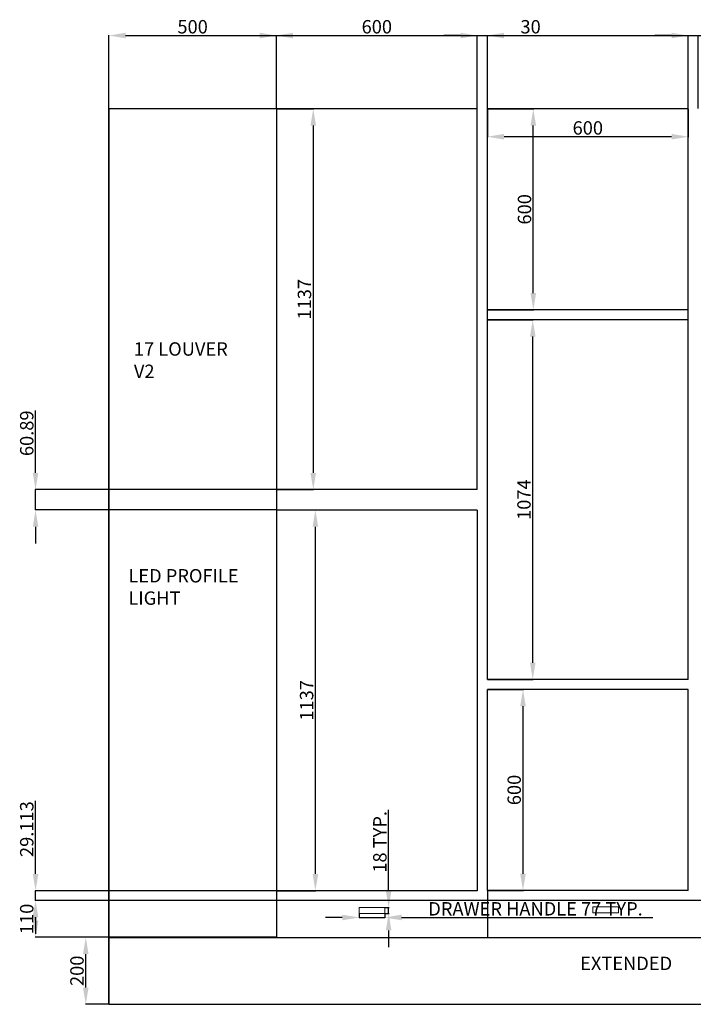
# Model space of a CAD drawing. Units: millimetres. Extents: x -2182 to 7969, y 257 to 4097.
# Tile 1 of 5: x -2182 to -171, y 508 to 3449. Entities that reach past the tile are written whole.
import ezdxf

# ---------------------------------------------------------------- set-up
doc = ezdxf.new("R2010")
doc.units = ezdxf.units.MM
for name, color, linetype, lineweight in [('A-ANNO-DIMS', 2, 'Continuous', 18), ('A-ANNO-TEXT', 3, 'Continuous', 18), ('A-ELEV', 7, 'Continuous', 25), ('A-FURN-HRDW', 8, 'Continuous', 18)]:
    doc.layers.add(name, color=color, linetype=linetype, lineweight=lineweight)
doc.styles.get("Standard").update_dxf_attribs({"font": 'arial.ttf'})
doc.dimstyles.new('ISO-25', dxfattribs={"dimtxt": 40, "dimasz": 50, "dimexe": 1.25, "dimexo": 0.625, "dimtad": 1, "dimtxsty": 'Standard', "dimcen": 2.5, "dimadec": 0, "dimazin": 0, "dimtfac": 1, "dimtmove": 0, "dimatfit": 3, "dimfxl": 1, "dimarcsym": 0})

# ---------------------------------------------------------------- blocks, each defined once
blk = doc.blocks.new('*D24')
at = {"layer": 'A-ANNO-DIMS', "color": 0, "lineweight": -2, "transparency": 16777216}
for p, q in [((-785.2, 1448.5), (-678.1, 1448.5)), ((-679.3, 898.5), (-679.3, 1398.5)), ((-785.2, 848.5), (-678.1, 848.5))]:
    blk.add_line(p, q, dxfattribs=at)
at = {"layer": 'A-ANNO-DIMS', "color": 0, "transparency": 16777216}
for points in [[(-687.7, 1398.5), (-671, 1398.5), (-679.3, 1448.5)], [(-687.7, 898.5), (-671, 898.5), (-679.3, 848.5)]]:
    blk.add_solid(points, dxfattribs=at)
at = {"layer": 'Defpoints', "color": 0, "transparency": 16777216}
for p in [(-785.8, 1448.5), (-679.3, 1448.5), (-785.8, 848.5)]:
    blk.add_point(p, dxfattribs=at)
at = {"layer": 'A-ANNO-DIMS', "color": 0, "transparency": 16777216, "insert": (-700.4, 1148.5), "char_height": 40, "attachment_point": 5, "rotation": 90}
blk.add_mtext('600', dxfattribs=at)
blk = doc.blocks.new('*D25')
at = {"layer": 'A-ANNO-DIMS', "color": 0, "lineweight": -2, "transparency": 16777216}
for p, q in [((-785.2, 2552.5), (-648.9, 2552.5)), ((-650.2, 1528.5), (-650.2, 2502.5)), ((-785.2, 1478.5), (-648.9, 1478.5))]:
    blk.add_line(p, q, dxfattribs=at)
at = {"layer": 'A-ANNO-DIMS', "color": 0, "transparency": 16777216}
for points in [[(-658.5, 2502.5), (-641.9, 2502.5), (-650.2, 2552.5)], [(-658.5, 1528.5), (-641.9, 1528.5), (-650.2, 1478.5)]]:
    blk.add_solid(points, dxfattribs=at)
at = {"layer": 'Defpoints', "color": 0, "transparency": 16777216}
for p in [(-785.8, 2552.5), (-650.2, 2552.5), (-785.8, 1478.5)]:
    blk.add_point(p, dxfattribs=at)
at = {"layer": 'A-ANNO-DIMS', "color": 0, "transparency": 16777216, "insert": (-671.2, 2015.5), "char_height": 40, "attachment_point": 5, "rotation": 90}
blk.add_mtext('1074', dxfattribs=at)
blk = doc.blocks.new('*D26')
at = {"layer": 'A-ANNO-DIMS', "color": 0, "lineweight": -2, "transparency": 16777216}
for p, q in [((-785.2, 3182.5), (-647.3, 3182.5)), ((-648.5, 2632.5), (-648.5, 3132.5)), ((-785.2, 2582.5), (-647.3, 2582.5))]:
    blk.add_line(p, q, dxfattribs=at)
at = {"layer": 'A-ANNO-DIMS', "color": 0, "transparency": 16777216}
for points in [[(-656.9, 3132.5), (-640.2, 3132.5), (-648.5, 3182.5)], [(-656.9, 2632.5), (-640.2, 2632.5), (-648.5, 2582.5)]]:
    blk.add_solid(points, dxfattribs=at)
at = {"layer": 'Defpoints', "color": 0, "transparency": 16777216}
for p in [(-785.8, 3182.5), (-648.5, 3182.5), (-785.8, 2582.5)]:
    blk.add_point(p, dxfattribs=at)
at = {"layer": 'A-ANNO-DIMS', "color": 0, "transparency": 16777216, "insert": (-669.6, 2882.5), "char_height": 40, "attachment_point": 5, "rotation": 90}
blk.add_mtext('600', dxfattribs=at)
blk = doc.blocks.new('*D27')
at = {"layer": 'A-ANNO-DIMS', "color": 0, "lineweight": -2, "transparency": 16777216}
for p, q in [((-785.8, 3181.8), (-785.8, 3098.1)), ((-185.8, 3181.8), (-185.8, 3098.1)), ((-235.8, 3099.3), (-735.8, 3099.3))]:
    blk.add_line(p, q, dxfattribs=at)
at = {"layer": 'A-ANNO-DIMS', "color": 0, "transparency": 16777216}
for points in [[(-735.8, 3107.7), (-735.8, 3091), (-785.8, 3099.3)], [(-235.8, 3107.7), (-235.8, 3091), (-185.8, 3099.3)]]:
    blk.add_solid(points, dxfattribs=at)
at = {"layer": 'Defpoints', "color": 0, "transparency": 16777216}
for p in [(-785.8, 3182.5), (-185.8, 3182.5), (-785.8, 3099.3)]:
    blk.add_point(p, dxfattribs=at)
at = {"layer": 'A-ANNO-DIMS', "color": 0, "transparency": 16777216, "insert": (-485.8, 3120.4), "char_height": 40, "attachment_point": 5}
blk.add_mtext('600', dxfattribs=at)
blk = doc.blocks.new('*D28')
at = {"layer": 'A-ANNO-DIMS', "color": 0, "lineweight": -2, "transparency": 16777216}
for p, q in [((-1415.2, 3182.5), (-1304.4, 3182.5)), ((-1305.6, 3132.5), (-1305.6, 2095.5)), ((-1415.2, 2045.5), (-1304.4, 2045.5))]:
    blk.add_line(p, q, dxfattribs=at)
at = {"layer": 'A-ANNO-DIMS', "color": 0, "transparency": 16777216}
for points in [[(-1314, 3132.5), (-1297.3, 3132.5), (-1305.6, 3182.5)], [(-1314, 2095.5), (-1297.3, 2095.5), (-1305.6, 2045.5)]]:
    blk.add_solid(points, dxfattribs=at)
at = {"layer": 'Defpoints', "color": 0, "transparency": 16777216}
for p in [(-1415.8, 3182.5), (-1415.8, 2045.5), (-1305.6, 2045.5)]:
    blk.add_point(p, dxfattribs=at)
at = {"layer": 'A-ANNO-DIMS', "color": 0, "transparency": 16777216, "insert": (-1326.7, 2614), "char_height": 40, "attachment_point": 5, "rotation": 90}
blk.add_mtext('1137', dxfattribs=at)
blk = doc.blocks.new('*D29')
at = {"layer": 'A-ANNO-DIMS', "color": 0, "lineweight": -2, "transparency": 16777216}
for p, q in [((-1415.2, 1984.6), (-1297.9, 1984.6)), ((-1299.2, 897.6), (-1299.2, 1934.6)), ((-1415.2, 847.6), (-1297.9, 847.6))]:
    blk.add_line(p, q, dxfattribs=at)
at = {"layer": 'A-ANNO-DIMS', "color": 0, "transparency": 16777216}
for points in [[(-1307.5, 1934.6), (-1290.8, 1934.6), (-1299.2, 1984.6)], [(-1307.5, 897.6), (-1290.8, 897.6), (-1299.2, 847.6)]]:
    blk.add_solid(points, dxfattribs=at)
at = {"layer": 'Defpoints', "color": 0, "transparency": 16777216}
for p in [(-1415.8, 1984.6), (-1299.2, 1984.6), (-1415.8, 847.6)]:
    blk.add_point(p, dxfattribs=at)
at = {"layer": 'A-ANNO-DIMS', "color": 0, "transparency": 16777216, "insert": (-1320.2, 1416.1), "char_height": 40, "attachment_point": 5, "rotation": 90}
blk.add_mtext('1137', dxfattribs=at)
blk = doc.blocks.new('*D30')
at = {"layer": 'A-ANNO-DIMS', "color": 0, "lineweight": -2, "transparency": 16777216}
for p, q in [((-1916.4, 708.5), (-1986.1, 708.5)), ((-1984.8, 558.5), (-1984.8, 658.5)), ((-1916.4, 508.5), (-1986.1, 508.5))]:
    blk.add_line(p, q, dxfattribs=at)
at = {"layer": 'A-ANNO-DIMS', "color": 0, "transparency": 16777216}
for points in [[(-1993.2, 658.5), (-1976.5, 658.5), (-1984.8, 708.5)], [(-1993.2, 558.5), (-1976.5, 558.5), (-1984.8, 508.5)]]:
    blk.add_solid(points, dxfattribs=at)
at = {"layer": 'Defpoints', "color": 0, "transparency": 16777216}
for p in [(-1984.8, 708.5), (-1915.8, 708.5), (-1915.8, 508.5)]:
    blk.add_point(p, dxfattribs=at)
at = {"layer": 'A-ANNO-DIMS', "color": 0, "transparency": 16777216, "insert": (-2005.9, 608.5), "char_height": 40, "attachment_point": 5, "rotation": 90}
blk.add_mtext('200', dxfattribs=at)
blk = doc.blocks.new('DRAWER-HANDLE')
blk.add_lwpolyline([(0, 18.2), (76.9, 18.2), (76.9, 0), (0, 0)], close=True)
blk = doc.blocks.new('*D62')
at = {"layer": 'A-ANNO-DIMS', "color": 0, "lineweight": -2, "transparency": 16777216}
for p, q in [((-1219, 767.7), (-1269, 767.7)), ((-1169, 778.7), (-1169, 766.5)), ((-1169, 767.7), (-1092.1, 767.7)), ((-1092.1, 778.7), (-1092.1, 766.5)), ((-1042.1, 767.7), (-292, 767.7))]:
    blk.add_line(p, q, dxfattribs=at)
at = {"layer": 'A-ANNO-DIMS', "color": 0, "transparency": 16777216}
for points in [[(-1219, 776.1), (-1219, 759.4), (-1169, 767.7)], [(-1042.1, 776.1), (-1042.1, 759.4), (-1092.1, 767.7)]]:
    blk.add_solid(points, dxfattribs=at)
at = {"layer": 'Defpoints', "color": 0, "transparency": 16777216}
for p in [(-1169, 779.3), (-1092.1, 779.3), (-1092.1, 767.7)]:
    blk.add_point(p, dxfattribs=at)
at = {"layer": 'A-ANNO-DIMS', "color": 0, "transparency": 16777216, "insert": (-642, 788.4), "char_height": 40, "attachment_point": 5}
blk.add_mtext('DRAWER HANDLE 77 TYP.', dxfattribs=at)
blk = doc.blocks.new('*D63')
at = {"layer": 'A-ANNO-DIMS', "color": 0, "lineweight": -2, "transparency": 16777216}
for p, q in [((-1080.5, 847.5), (-1080.5, 1089.7)), ((-1091.4, 797.5), (-1079.3, 797.5)), ((-1080.5, 779.3), (-1080.5, 797.5)), ((-1091.4, 779.3), (-1079.3, 779.3)), ((-1080.5, 729.3), (-1080.5, 679.3))]:
    blk.add_line(p, q, dxfattribs=at)
at = {"layer": 'A-ANNO-DIMS', "color": 0, "transparency": 16777216}
for points in [[(-1088.9, 847.5), (-1072.2, 847.5), (-1080.5, 797.5)], [(-1088.9, 729.3), (-1072.2, 729.3), (-1080.5, 779.3)]]:
    blk.add_solid(points, dxfattribs=at)
at = {"layer": 'Defpoints', "color": 0, "transparency": 16777216}
for p in [(-1092.1, 797.5), (-1080.5, 797.5), (-1092.1, 779.3)]:
    blk.add_point(p, dxfattribs=at)
at = {"layer": 'A-ANNO-DIMS', "color": 0, "transparency": 16777216, "insert": (-1101.6, 993.6), "char_height": 40, "attachment_point": 5, "rotation": 90}
blk.add_mtext('18 TYP.', dxfattribs=at)
blk = doc.blocks.new('*D64')
at = {"layer": 'A-ANNO-DIMS', "color": 0, "lineweight": -2, "transparency": 16777216}
for p, q in [((-1915.8, 509.1), (-1915.8, 3402.7)), ((-1865.8, 3401.5), (2193.2, 3401.5)), ((2243.2, 3183.1), (2243.2, 3402.7))]:
    blk.add_line(p, q, dxfattribs=at)
at = {"layer": 'A-ANNO-DIMS', "color": 0, "transparency": 16777216}
for points in [[(-1865.8, 3409.8), (-1865.8, 3393.1), (-1915.8, 3401.5)], [(2193.2, 3409.8), (2193.2, 3393.1), (2243.2, 3401.5)]]:
    blk.add_solid(points, dxfattribs=at)
at = {"layer": 'Defpoints', "color": 0, "transparency": 16777216}
for p in [(2243.2, 3401.5), (2243.2, 3182.5), (-1915.8, 508.5)]:
    blk.add_point(p, dxfattribs=at)
at = {"layer": 'A-ANNO-DIMS', "color": 0, "transparency": 16777216, "insert": (163.7, 3422.5), "char_height": 40, "attachment_point": 5}
blk.add_mtext('4159', dxfattribs=at)
blk = doc.blocks.new('*D66')
at = {"layer": 'A-ANNO-DIMS', "color": 0, "lineweight": -2, "transparency": 16777216}
for p, q in [((-1915.8, 3183.1), (-1915.8, 3402.7)), ((-1865.8, 3401.5), (-1465.8, 3401.5)), ((-1415.8, 3183.1), (-1415.8, 3402.7))]:
    blk.add_line(p, q, dxfattribs=at)
at = {"layer": 'A-ANNO-DIMS', "color": 0, "transparency": 16777216}
for points in [[(-1865.8, 3409.8), (-1865.8, 3393.1), (-1915.8, 3401.5)], [(-1465.8, 3409.8), (-1465.8, 3393.1), (-1415.8, 3401.5)]]:
    blk.add_solid(points, dxfattribs=at)
at = {"layer": 'Defpoints', "color": 0, "transparency": 16777216}
for p in [(-1415.8, 3401.5), (-1915.8, 3182.5), (-1415.8, 3182.5)]:
    blk.add_point(p, dxfattribs=at)
at = {"layer": 'A-ANNO-DIMS', "color": 0, "transparency": 16777216, "insert": (-1665.8, 3422.5), "char_height": 40, "attachment_point": 5}
blk.add_mtext('500', dxfattribs=at)
blk = doc.blocks.new('*D67')
at = {"layer": 'A-ANNO-DIMS', "color": 0, "lineweight": -2, "transparency": 16777216}
for p, q in [((-1415.8, 3183.1), (-1415.8, 3402.7)), ((-1365.8, 3401.5), (-865.8, 3401.5)), ((-815.8, 3183.1), (-815.8, 3402.7))]:
    blk.add_line(p, q, dxfattribs=at)
at = {"layer": 'A-ANNO-DIMS', "color": 0, "transparency": 16777216}
for points in [[(-1365.8, 3409.8), (-1365.8, 3393.1), (-1415.8, 3401.5)], [(-865.8, 3409.8), (-865.8, 3393.1), (-815.8, 3401.5)]]:
    blk.add_solid(points, dxfattribs=at)
at = {"layer": 'Defpoints', "color": 0, "transparency": 16777216}
for p in [(-815.8, 3401.5), (-1415.8, 3182.5), (-815.8, 3182.5)]:
    blk.add_point(p, dxfattribs=at)
at = {"layer": 'A-ANNO-DIMS', "color": 0, "transparency": 16777216, "insert": (-1115.8, 3422.5), "char_height": 40, "attachment_point": 5}
blk.add_mtext('600', dxfattribs=at)
blk = doc.blocks.new('*D68')
at = {"layer": 'A-ANNO-DIMS', "color": 0, "lineweight": -2, "transparency": 16777216}
for p, q in [((-865.8, 3401.5), (-915.8, 3401.5)), ((-815.8, 3183.1), (-815.8, 3402.7)), ((-815.8, 3401.5), (-785.8, 3401.5)), ((-785.8, 3183.1), (-785.8, 3402.7)), ((-735.8, 3401.5), (-627.4, 3401.5))]:
    blk.add_line(p, q, dxfattribs=at)
at = {"layer": 'A-ANNO-DIMS', "color": 0, "transparency": 16777216}
for points in [[(-865.8, 3409.8), (-865.8, 3393.1), (-815.8, 3401.5)], [(-735.8, 3409.8), (-735.8, 3393.1), (-785.8, 3401.5)]]:
    blk.add_solid(points, dxfattribs=at)
at = {"layer": 'Defpoints', "color": 0, "transparency": 16777216}
for p in [(-785.8, 3401.5), (-815.8, 3182.5), (-785.8, 3182.5)]:
    blk.add_point(p, dxfattribs=at)
at = {"layer": 'A-ANNO-DIMS', "color": 0, "transparency": 16777216, "insert": (-656.6, 3422.5), "char_height": 40, "attachment_point": 5}
blk.add_mtext('30', dxfattribs=at)
blk = doc.blocks.new('*D69')
at = {"layer": 'A-ANNO-DIMS', "color": 0, "lineweight": -2, "transparency": 16777216}
for p, q in [((-235.8, 3401.5), (-285.8, 3401.5)), ((-185.8, 3183.1), (-185.8, 3402.7)), ((-185.8, 3401.5), (-155.8, 3401.5)), ((-155.8, 3183.1), (-155.8, 3402.7)), ((-105.8, 3401.5), (2.6, 3401.5))]:
    blk.add_line(p, q, dxfattribs=at)
at = {"layer": 'A-ANNO-DIMS', "color": 0, "transparency": 16777216}
for points in [[(-235.8, 3409.8), (-235.8, 3393.1), (-185.8, 3401.5)], [(-105.8, 3409.8), (-105.8, 3393.1), (-155.8, 3401.5)]]:
    blk.add_solid(points, dxfattribs=at)
at = {"layer": 'Defpoints', "color": 0, "transparency": 16777216}
for p in [(-155.8, 3401.5), (-185.8, 3182.5), (-155.8, 3182.5)]:
    blk.add_point(p, dxfattribs=at)
at = {"layer": 'A-ANNO-DIMS', "color": 0, "transparency": 16777216, "insert": (-26.6, 3422.5), "char_height": 40, "attachment_point": 5}
blk.add_mtext('30', dxfattribs=at)
blk = doc.blocks.new('*D74')
at = {"layer": 'A-ANNO-DIMS', "color": 0, "lineweight": -2, "transparency": 16777216}
for p, q in [((-1416.4, 818.5), (-2136.1, 818.5)), ((-2134.8, 758.5), (-2134.8, 768.5)), ((-1416.4, 708.5), (-2136.1, 708.5))]:
    blk.add_line(p, q, dxfattribs=at)
at = {"layer": 'A-ANNO-DIMS', "color": 0, "transparency": 16777216}
for points in [[(-2143.1, 768.5), (-2126.5, 768.5), (-2134.8, 818.5)], [(-2143.1, 758.5), (-2126.5, 758.5), (-2134.8, 708.5)]]:
    blk.add_solid(points, dxfattribs=at)
at = {"layer": 'Defpoints', "color": 0, "transparency": 16777216}
for p in [(-2134.8, 818.5), (-1415.8, 818.5), (-1415.8, 708.5)]:
    blk.add_point(p, dxfattribs=at)
at = {"layer": 'A-ANNO-DIMS', "color": 0, "transparency": 16777216, "insert": (-2155.9, 763.5), "char_height": 40, "attachment_point": 5, "rotation": 90}
blk.add_mtext('110', dxfattribs=at)
blk = doc.blocks.new('*D75')
at = {"layer": 'A-ANNO-DIMS', "color": 0, "lineweight": -2, "transparency": 16777216}
for p, q in [((-2134.8, 897.6), (-2134.8, 1115.6)), ((-1416.4, 847.6), (-2136.1, 847.6)), ((-2134.8, 818.5), (-2134.8, 847.6)), ((-1416.4, 818.5), (-2136.1, 818.5)), ((-2134.8, 768.5), (-2134.8, 718.5))]:
    blk.add_line(p, q, dxfattribs=at)
at = {"layer": 'A-ANNO-DIMS', "color": 0, "transparency": 16777216}
for points in [[(-2143.1, 897.6), (-2126.5, 897.6), (-2134.8, 847.6)], [(-2143.1, 768.5), (-2126.5, 768.5), (-2134.8, 818.5)]]:
    blk.add_solid(points, dxfattribs=at)
at = {"layer": 'Defpoints', "color": 0, "transparency": 16777216}
for p in [(-2134.8, 847.6), (-1415.8, 847.6), (-1415.8, 818.5)]:
    blk.add_point(p, dxfattribs=at)
at = {"layer": 'A-ANNO-DIMS', "color": 0, "transparency": 16777216, "insert": (-2155.9, 1031.6), "char_height": 40, "attachment_point": 5, "rotation": 90}
blk.add_mtext('29.113', dxfattribs=at)
blk = doc.blocks.new('*D76')
at = {"layer": 'A-ANNO-DIMS', "color": 0, "lineweight": -2, "transparency": 16777216}
for p, q in [((-2134.8, 2095.5), (-2134.8, 2282)), ((-1416.4, 2045.5), (-2136.1, 2045.5)), ((-2134.8, 1984.6), (-2134.8, 2045.5)), ((-1416.4, 1984.6), (-2136.1, 1984.6)), ((-2134.8, 1934.6), (-2134.8, 1884.6))]:
    blk.add_line(p, q, dxfattribs=at)
at = {"layer": 'A-ANNO-DIMS', "color": 0, "transparency": 16777216}
for points in [[(-2143.1, 2095.5), (-2126.5, 2095.5), (-2134.8, 2045.5)], [(-2143.1, 1934.6), (-2126.5, 1934.6), (-2134.8, 1984.6)]]:
    blk.add_solid(points, dxfattribs=at)
at = {"layer": 'Defpoints', "color": 0, "transparency": 16777216}
for p in [(-2134.8, 2045.5), (-1415.8, 2045.5), (-1415.8, 1984.6)]:
    blk.add_point(p, dxfattribs=at)
at = {"layer": 'A-ANNO-DIMS', "color": 0, "transparency": 16777216, "insert": (-2155.9, 2213.7), "char_height": 40, "attachment_point": 5, "rotation": 90}
blk.add_mtext('60.89', dxfattribs=at)

msp = doc.modelspace()

# ---------------------------------------------------------------- linework, layer by layer
at = {"layer": 'A-ELEV'}
for p, q in [((-815.8106, 3182.4543), (-1915.8106, 3182.4543)), ((-1915.8106, 3182.4543), (-1915.8106, 508.4543)), ((-1415.8106, 3182.4543), (-1415.8106, 708.4543)), ((-815.8106, 2045.4543), (-815.8106, 3182.4543)), ((-185.8106, 3182.4543), (-785.8106, 3182.4543)), ((-785.8106, 1478.4543), (-785.8106, 3182.4543)), ((-185.8106, 1478.4543), (-185.8106, 3182.4543)), ((-185.8106, 2582.4543), (-785.8106, 2582.4543)), ((-185.8106, 2552.4543), (-785.8106, 2552.4543)), ((-815.8106, 2045.4543), (-1415.8106, 2045.4543)), ((-815.8106, 1984.5674), (-1415.8106, 1984.5674)), ((-815.8106, 1984.5674), (-815.8106, 847.5674)), ((-185.8106, 1478.4543), (-785.8106, 1478.4543)), ((-785.8106, 848.4543), (-785.8106, 1448.4543)), ((-185.8106, 1448.4543), (-785.8106, 1448.4543)), ((-185.8106, 848.4543), (-185.8106, 1448.4543)), ((-815.8106, 847.5674), (-1415.8106, 847.5674)), ((-185.8106, 848.4543), (-785.8106, 848.4543)), ((-785.8106, 848.4543), (-785.8106, 708.4543)), ((1093.1894, 818.4543), (-1415.8106, 818.4543)), ((-1915.8106, 708.4543), (1093.1894, 708.4543)), ((-1915.8106, 508.4543), (2193.1894, 508.4543))]:
    msp.add_line(p, q, dxfattribs=at)

# ---------------------------------------------------------------- block references
at = {"layer": 'A-FURN-HRDW'}
for p in [(-1168.95, 779.276), (-471.1747, 781.1971)]:
    msp.add_blockref('DRAWER-HANDLE', p, dxfattribs=at)

# ---------------------------------------------------------------- texts
at = {"layer": 'A-ANNO-TEXT', "char_height": 40, "width": 482.986246, "attachment_point": 1}
for s, insert in [('17 LOUVER \\P     V2', (-1841.1455, 2485.3775)), ('LED PROFILE \\PLIGHT', (-1857.5525, 1808.1376)), ('EXTENDED', (-508.7573, 650.6308))]:
    msp.add_mtext(s, dxfattribs=dict(at, insert=insert))

# ---------------------------------------------------------------- dimensions: what is measured, and where the dimension line sits
at = {"layer": 'A-ANNO-DIMS'}
for base, p1, p2, override, picture, middle in [((2243.1894, 3401.4543), (-1915.8106, 508.4543), (2243.1894, 3182.4543), {"dimdec": 0, "dimlfac": 1, "dimrnd": 0, "dimzin": 0, "dimdsep": 46, "dimlunit": 2}, '*D64', (163.6894, 3422.5022)), ((-1415.8106, 3401.4543), (-1915.8106, 3182.4543), (-1415.8106, 3182.4543), {"dimdec": 0, "dimlfac": 1, "dimrnd": 0, "dimzin": 0, "dimdsep": 46, "dimlunit": 2}, '*D66', (-1665.8106, 3422.5022)), ((-815.8106, 3401.4543), (-1415.8106, 3182.4543), (-815.8106, 3182.4543), {"dimdec": 0, "dimlfac": 1, "dimrnd": 0, "dimzin": 0, "dimdsep": 46, "dimlunit": 2}, '*D67', (-1115.8106, 3422.5022)), ((-785.8106, 3401.4543), (-815.8106, 3182.4543), (-785.8106, 3182.4543), {"dimdec": 0, "dimlfac": 1, "dimrnd": 0, "dimzin": 0, "dimdsep": 46, "dimlunit": 2}, '*D68', (-656.6181, 3422.5159)), ((-155.8106, 3401.4543), (-185.8106, 3182.4543), (-155.8106, 3182.4543), {"dimdec": 0, "dimlfac": 1, "dimrnd": 0, "dimzin": 0, "dimdsep": 46, "dimlunit": 2}, '*D69', (-26.6181, 3422.5159)), ((-785.8106, 3099.3254), (-185.8106, 3182.4543), (-785.8106, 3182.4543), {"dimclrd": 0, "dimclre": 0, "dimclrt": 0}, '*D27', (-485.8106, 3120.3733))]:
    dim = msp.add_linear_dim(base=base, p1=p1, p2=p2, dimstyle='ISO-25', override=override, dxfattribs=at)
    dim.commit()
    dim.dimension.update_dxf_attribs({"geometry": picture, "text_midpoint": middle})
for base, p1, p2, override, picture, middle in [((-1305.6276, 2045.4543), (-1415.8106, 3182.4543), (-1415.8106, 2045.4543), {"dimclrd": 0, "dimclre": 0, "dimclrt": 0}, '*D28', (-1326.6891, 2613.9543)), ((-650.1896, 2552.4543), (-785.8106, 1478.4543), (-785.8106, 2552.4543), {"dimclrd": 0, "dimclre": 0, "dimclrt": 0}, '*D25', (-671.2375, 2015.4543)), ((-2134.8106, 2045.4543), (-1415.8106, 1984.5674), (-1415.8106, 2045.4543), {"dimdec": 2, "dimlfac": 1, "dimrnd": 0, "dimzin": 0, "dimdsep": 46, "dimlunit": 2}, '*D76', (-2155.8585, 2213.7191)), ((-1299.1592, 1984.5674), (-1415.8106, 847.5674), (-1415.8106, 1984.5674), {"dimclrd": 0, "dimclre": 0, "dimclrt": 0}, '*D29', (-1320.2208, 1416.0674)), ((-679.3428, 1448.4543), (-785.8106, 848.4543), (-785.8106, 1448.4543), {"dimclrd": 0, "dimclre": 0, "dimclrt": 0}, '*D24', (-700.3907, 1148.4543)), ((-2134.8106, 847.5674), (-1415.8106, 818.4543), (-1415.8106, 847.5674), {"dimdec": 3, "dimlfac": 1, "dimrnd": 0, "dimzin": 0, "dimdsep": 46, "dimlunit": 2}, '*D75', (-2155.8722, 1031.5622)), ((-2134.8106, 818.4543), (-1415.8106, 708.4543), (-1415.8106, 818.4543), {"dimdec": 0, "dimlfac": 1, "dimrnd": 0, "dimzin": 0, "dimdsep": 46, "dimlunit": 2}, '*D74', (-2155.8585, 763.4543)), ((-1984.8202, 708.4543), (-1915.8106, 508.4543), (-1915.8106, 708.4543), {"dimclrd": 0, "dimclre": 0, "dimclrt": 0}, '*D30', (-2005.8682, 608.4543))]:
    dim = msp.add_linear_dim(base=base, p1=p1, p2=p2, angle=90, dimstyle='ISO-25', override=override, dxfattribs=at)
    dim.commit()
    dim.dimension.update_dxf_attribs({"geometry": picture, "text_midpoint": middle})
dim = msp.add_linear_dim(base=(-648.5188, 3182.4543), p1=(-785.8106, 2582.4543), p2=(-785.8106, 3182.4543), angle=90, dimstyle='ISO-25', override={"dimclrd": 0, "dimclre": 0, "dimclrt": 0}, dxfattribs=at)
dim.commit()
dim.dimension.update_dxf_attribs({"geometry": '*D26', "text_midpoint": (-648.5188, 2882.4543), "dimtype": 160})
dim = msp.add_linear_dim(base=(-1080.5256, 797.5255), p1=(-1092.0592, 779.2758), p2=(-1092.0592, 797.5255), angle=90, text='<> TYP.', dimstyle='ISO-25', override={"dimdec": 0, "dimrnd": 0, "dimzin": 0, "dimlunit": 2}, dxfattribs=at)
dim.commit()
dim.dimension.update_dxf_attribs({"geometry": '*D63', "text_midpoint": (-1101.5735, 993.6212)})
dim = msp.add_linear_dim(base=(-1092.0592, 767.7422), p1=(-1168.9501, 779.2758), p2=(-1092.0592, 779.2758), text='DRAWER HANDLE <> TYP.', dimstyle='ISO-25', override={"dimdec": 0, "dimrnd": 0, "dimzin": 0, "dimlunit": 2}, dxfattribs=at)
dim.commit()
dim.dimension.update_dxf_attribs({"geometry": '*D62', "text_midpoint": (-642.0345, 788.3809)})

doc.saveas('drawing.dxf')
